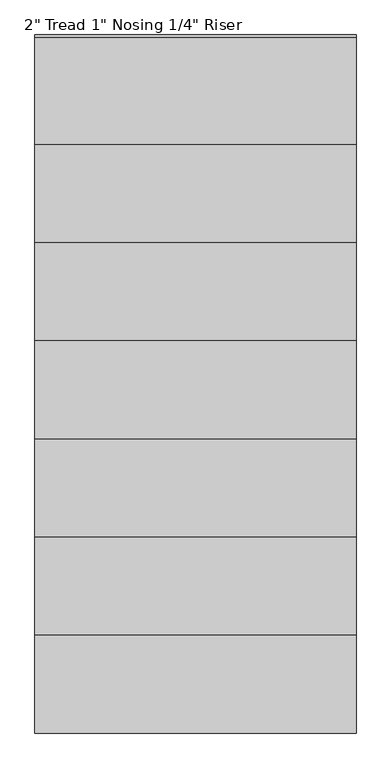
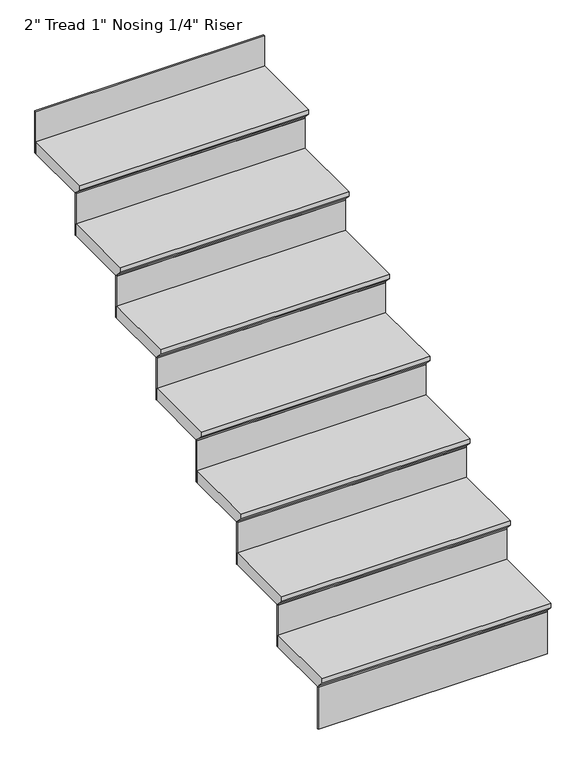
"""IFC4 building model written with IfcOpenShell, lengths in millimetres: stair flight geometry."""

from ifc_helpers import new_model, si_unit, frame, origin, place, context, project, spatial, polyline, outline, extrude, source, transform, mapped, element, save


def stair_flight_d9814c51(model_context):
    return source(origin(), model_context, "Body", "SweptSolid", [
        extrude(outline(polyline([(-3538.5064015, 2565.4), (-3233.7064015, 2565.4), (-3233.7064015, 2514.6), (-3513.1064015, 2514.6), (-3513.1064015, 2520.95), (-3538.5064015, 2546.35), (-3538.5064015, 2565.4)])), frame((-4591.1993763, 0.0, 0.0), z_axis=(1.0, 0.0, 0.0), x_axis=(0.0, 1.0, 0.0)), (0.0, 0.0, 1.0), 914.4),
        extrude(outline(polyline([(-3676.7993763, -3506.7564015), (-3676.7993763, -3513.1064015), (-4591.1993763, -3513.1064015), (-4591.1993763, -3506.7564015), (-3676.7993763, -3506.7564015)])), frame((0.0, 0.0, 2336.8), z_axis=(0.0, 0.0, 1.0), x_axis=(1.0, 0.0, 0.0)), (0.0, 0.0, 1.0), 177.8),
        extrude(outline(polyline([(-3676.7993763, -3227.3564015), (-3676.7993763, -3233.7064015), (-4591.1993763, -3233.7064015), (-4591.1993763, -3227.3564015), (-3676.7993763, -3227.3564015)])), frame((0.0, 0.0, 2514.6), z_axis=(0.0, 0.0, 1.0), x_axis=(1.0, 0.0, 0.0)), (0.0, 0.0, 1.0), 177.8),
        extrude(outline(polyline([(-3259.1064015, 2743.2), (-2954.3064015, 2743.2), (-2954.3064015, 2692.4), (-3233.7064015, 2692.4), (-3233.7064015, 2698.75), (-3259.1064015, 2724.15), (-3259.1064015, 2743.2)])), frame((-4591.1993763, 0.0, 0.0), z_axis=(1.0, 0.0, 0.0), x_axis=(0.0, 1.0, 0.0)), (0.0, 0.0, 1.0), 914.4),
        extrude(outline(polyline([(-3676.7993763, -2947.9564015), (-3676.7993763, -2954.3064015), (-4591.1993763, -2954.3064015), (-4591.1993763, -2947.9564015), (-3676.7993763, -2947.9564015)])), frame((0.0, 0.0, 2692.4), z_axis=(0.0, 0.0, 1.0), x_axis=(1.0, 0.0, 0.0)), (0.0, 0.0, 1.0), 177.8),
        extrude(outline(polyline([(-2979.7064015, 2921.0), (-2674.9064015, 2921.0), (-2674.9064015, 2870.2), (-2954.3064015, 2870.2), (-2954.3064015, 2876.55), (-2979.7064015, 2901.95), (-2979.7064015, 2921.0)])), frame((-4591.1993763, 0.0, 0.0), z_axis=(1.0, 0.0, 0.0), x_axis=(0.0, 1.0, 0.0)), (0.0, 0.0, 1.0), 914.4),
        extrude(outline(polyline([(-3676.7993763, -2668.5564015), (-3676.7993763, -2674.9064015), (-4591.1993763, -2674.9064015), (-4591.1993763, -2668.5564015), (-3676.7993763, -2668.5564015)])), frame((0.0, 0.0, 2870.2), z_axis=(0.0, 0.0, 1.0), x_axis=(1.0, 0.0, 0.0)), (0.0, 0.0, 1.0), 177.8),
        extrude(outline(polyline([(-2700.3064015, 3098.8), (-2395.5064015, 3098.8), (-2395.5064015, 3048.0), (-2674.9064015, 3048.0), (-2674.9064015, 3054.35), (-2700.3064015, 3079.75), (-2700.3064015, 3098.8)])), frame((-4591.1993763, 0.0, 0.0), z_axis=(1.0, 0.0, 0.0), x_axis=(0.0, 1.0, 0.0)), (0.0, 0.0, 1.0), 914.4),
        extrude(outline(polyline([(-3676.7993763, -2389.1564015), (-3676.7993763, -2395.5064015), (-4591.1993763, -2395.5064015), (-4591.1993763, -2389.1564015), (-3676.7993763, -2389.1564015)])), frame((0.0, 0.0, 3048.0), z_axis=(0.0, 0.0, 1.0), x_axis=(1.0, 0.0, 0.0)), (0.0, 0.0, 1.0), 177.8),
        extrude(outline(polyline([(-2420.9064015, 3276.6), (-2116.1064015, 3276.6), (-2116.1064015, 3225.8), (-2395.5064015, 3225.8), (-2395.5064015, 3232.15), (-2420.9064015, 3257.55), (-2420.9064015, 3276.6)])), frame((-4591.1993763, 0.0, 0.0), z_axis=(1.0, 0.0, 0.0), x_axis=(0.0, 1.0, 0.0)), (0.0, 0.0, 1.0), 914.4),
        extrude(outline(polyline([(-3676.7993763, -2109.7564015), (-3676.7993763, -2116.1064015), (-4591.1993763, -2116.1064015), (-4591.1993763, -2109.7564015), (-3676.7993763, -2109.7564015)])), frame((0.0, 0.0, 3225.8), z_axis=(0.0, 0.0, 1.0), x_axis=(1.0, 0.0, 0.0)), (0.0, 0.0, 1.0), 177.8),
        extrude(outline(polyline([(-2141.5064015, 3454.4), (-1836.7064015, 3454.4), (-1836.7064015, 3403.6), (-2116.1064015, 3403.6), (-2116.1064015, 3409.95), (-2141.5064015, 3435.35), (-2141.5064015, 3454.4)])), frame((-4591.1993763, 0.0, 0.0), z_axis=(1.0, 0.0, 0.0), x_axis=(0.0, 1.0, 0.0)), (0.0, 0.0, 1.0), 914.4),
        extrude(outline(polyline([(-3676.7993763, -1830.3564015), (-3676.7993763, -1836.7064015), (-4591.1993763, -1836.7064015), (-4591.1993763, -1830.3564015), (-3676.7993763, -1830.3564015)])), frame((0.0, 0.0, 3403.6), z_axis=(0.0, 0.0, 1.0), x_axis=(1.0, 0.0, 0.0)), (0.0, 0.0, 1.0), 177.8),
        extrude(outline(polyline([(-3676.7993763, -1550.9564015), (-3676.7993763, -1557.3064015), (-4591.1993763, -1557.3064015), (-4591.1993763, -1550.9564015), (-3676.7993763, -1550.9564015)])), frame((0.0, 0.0, 3581.4), z_axis=(0.0, 0.0, 1.0), x_axis=(1.0, 0.0, 0.0)), (0.0, 0.0, 1.0), 177.8),
        extrude(outline(polyline([(-1862.1064015, 3632.2), (-1557.3064015, 3632.2), (-1557.3064015, 3581.4), (-1836.7064015, 3581.4), (-1836.7064015, 3587.75), (-1862.1064015, 3613.15), (-1862.1064015, 3632.2)])), frame((-4591.1993763, 0.0, 0.0), z_axis=(1.0, 0.0, 0.0), x_axis=(0.0, 1.0, 0.0)), (0.0, 0.0, 1.0), 914.4),
    ])


if __name__ == "__main__":
    model = new_model("IFC4")
    model_context = context("Model", 3, world=origin())
    ifc_project = project(units=[si_unit("LENGTHUNIT", "METRE", prefix="MILLI")], contexts=[model_context])
    site = spatial("IfcSite", under=ifc_project)
    building = spatial("IfcBuilding", under=site)
    placement = place(None, origin())
    stair_flight_shape = stair_flight_d9814c51(model_context)
    element("IfcStairFlight", 1, ObjectType="2\" Tread 1\" Nosing 1/4\" Riser", at=placement, inside=building, context=model_context, shape_type="MappedRepresentation", body=[
        mapped(stair_flight_shape, transform((0.0, 0.0, 0.0), x_axis=(1.0, 0.0, 0.0), y_axis=(0.0, 1.0, 0.0), z_axis=(0.0, 0.0, 1.0))),
    ])
    save(model, "model.ifc")
